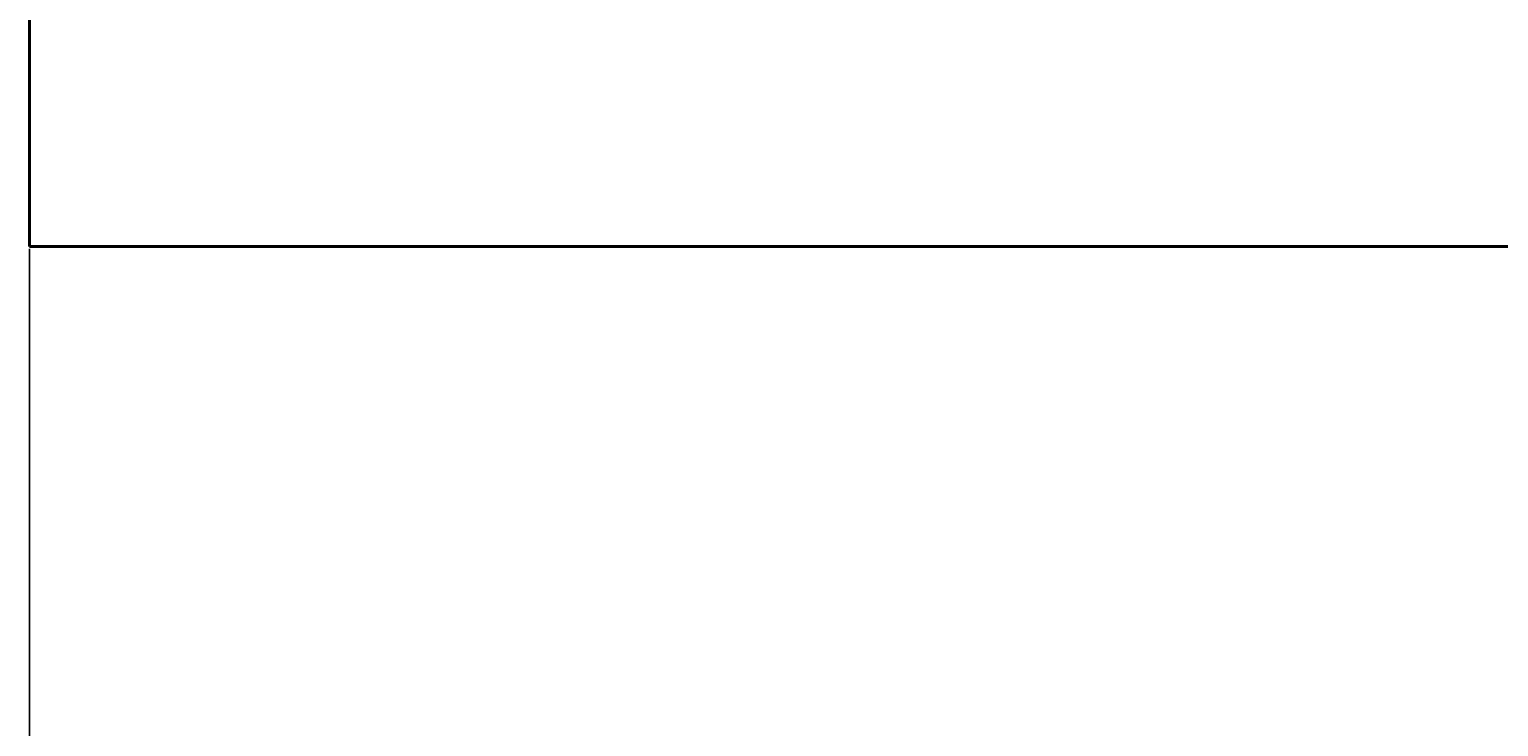
# Model space of a CAD drawing. Units: inches. Extents: x -301 to 715, y -607 to 364.
# Tile 55 of 141: x -205 to -164, y -237 to -218. Entities that reach past the tile are written whole.
import ezdxf

# ---------------------------------------------------------------- set-up
doc = ezdxf.new("R2010")
doc.units = ezdxf.units.IN
doc.header["$MEASUREMENT"] = 0
doc.layers.add('A-ANNO-DIMS', color=2, linetype='Continuous', lineweight=18)
doc.layers.add('A-WALL', color=3, linetype='Continuous', lineweight=40)
doc.styles.get("Standard").update_dxf_attribs({"font": 'arial.ttf'})
doc.dimstyles.get("Standard").update_dxf_attribs({"dimtxt": 0.18, "dimasz": 0.18, "dimexe": 0.18, "dimexo": 0.0625, "dimgap": 0.09, "dimtad": 0, "dimtih": 1, "dimtoh": 1, "dimdec": 1, "dimzin": 0, "dimdsep": 46, "dimlunit": 4, "dimtxsty": 'Standard', "dimcen": 0.09, "dimclrd": 3, "dimclre": 4, "dimclrt": 6, "dimadec": 0, "dimazin": 0, "dimtfac": 1, "dimtdec": 1, "dimtofl": 0, "dimtmove": 0, "dimatfit": 3, "dimfxl": 1, "dimtfill": 2, "dimtfillclr": 51, "dimtolj": 1, "dimtzin": 0, "dimarcsym": 0})

# ---------------------------------------------------------------- blocks, each defined once
blk = doc.blocks.new('*D146')
at = {"layer": 'A-ANNO-DIMS', "color": 4, "lineweight": -2, "transparency": 16777216}
for p, q in [((-204.603, -223.88), (-204.603, -296.865)), ((-143.603, -223.88), (-143.603, -296.865))]:
    blk.add_line(p, q, dxfattribs=at)
at = {"layer": 'A-ANNO-DIMS', "color": 3, "lineweight": -2, "transparency": 16777216}
for p, q in [((-204.423, -296.685), (-174.433, -296.685)), ((-143.783, -296.685), (-173.774, -296.685))]:
    blk.add_line(p, q, dxfattribs=at)
at = {"layer": 'A-ANNO-DIMS', "color": 3, "transparency": 16777216}
for points in [[(-204.423, -296.655), (-204.423, -296.715), (-204.603, -296.685)], [(-143.783, -296.655), (-143.783, -296.715), (-143.603, -296.685)]]:
    blk.add_solid(points, dxfattribs=at)
at = {"layer": 'Defpoints', "color": 0, "transparency": 16777216}
for p in [(-204.603, -223.818), (-143.603, -223.818), (-143.603, -296.685)]:
    blk.add_point(p, dxfattribs=at)
at = {"layer": 'A-ANNO-DIMS', "color": 6, "transparency": 16777216, "insert": (-174.103, -296.685), "char_height": 0.18, "attachment_point": 5, "bg_fill": 1, "box_fill_scale": 1.25, "bg_fill_color": 51, "bg_fill_transparency": 0}
blk.add_mtext('\\A1;5\'-1"', dxfattribs=at)
blk = doc.blocks.new('*D151')
at = {"layer": 'A-ANNO-DIMS', "color": 4, "lineweight": -2, "transparency": 16777216}
for p, q in [((-204.603, -223.755), (-204.603, 359.612)), ((-45.603, -214.755), (-45.603, 359.612))]:
    blk.add_line(p, q, dxfattribs=at)
at = {"layer": 'A-ANNO-DIMS', "color": 3, "lineweight": -2, "transparency": 16777216}
for p, q in [((-204.423, 359.432), (-125.494, 359.432)), ((-45.783, 359.432), (-124.713, 359.432))]:
    blk.add_line(p, q, dxfattribs=at)
at = {"layer": 'A-ANNO-DIMS', "color": 3, "transparency": 16777216}
for points in [[(-204.423, 359.462), (-204.423, 359.402), (-204.603, 359.432)], [(-45.783, 359.462), (-45.783, 359.402), (-45.603, 359.432)]]:
    blk.add_solid(points, dxfattribs=at)
at = {"layer": 'Defpoints', "color": 0, "transparency": 16777216}
for p in [(-45.603, 359.432), (-45.603, -214.818), (-204.603, -223.818)]:
    blk.add_point(p, dxfattribs=at)
at = {"layer": 'A-ANNO-DIMS', "color": 6, "transparency": 16777216, "insert": (-125.103, 359.432), "char_height": 0.18, "attachment_point": 5, "bg_fill": 1, "box_fill_scale": 1.25, "bg_fill_color": 51, "bg_fill_transparency": 0}
blk.add_mtext('\\A1;13\'-3"', dxfattribs=at)

msp = doc.modelspace()

# ---------------------------------------------------------------- linework, layer by layer
at = {"layer": 'A-WALL'}
for p, q in [((-204.603, -67.318), (-204.603, -223.818)), ((-204.603, -223.818), (-45.603, -223.818))]:
    msp.add_line(p, q, dxfattribs=at)

# ---------------------------------------------------------------- dimensions: what is measured, and where the dimension line sits
at = {"layer": 'A-ANNO-DIMS'}
for base, p2, picture, middle in [((-45.603, 359.432), (-45.603, -214.818), '*D151', (-125.103, 359.432)), ((-143.603, -296.685), (-143.603, -223.818), '*D146', (-174.103, -296.685))]:
    dim = msp.add_linear_dim(base=base, p1=(-204.603, -223.818), p2=p2, dimstyle='Standard', override={"dimdec": 1, "dimlfac": 1, "dimrnd": 0, "dimzin": 1, "dimdsep": 46, "dimlunit": 4, "dimfrac": 2}, dxfattribs=at)
    dim.commit()
    dim.dimension.update_dxf_attribs({"geometry": picture, "text_midpoint": middle})

doc.saveas('drawing.dxf')
